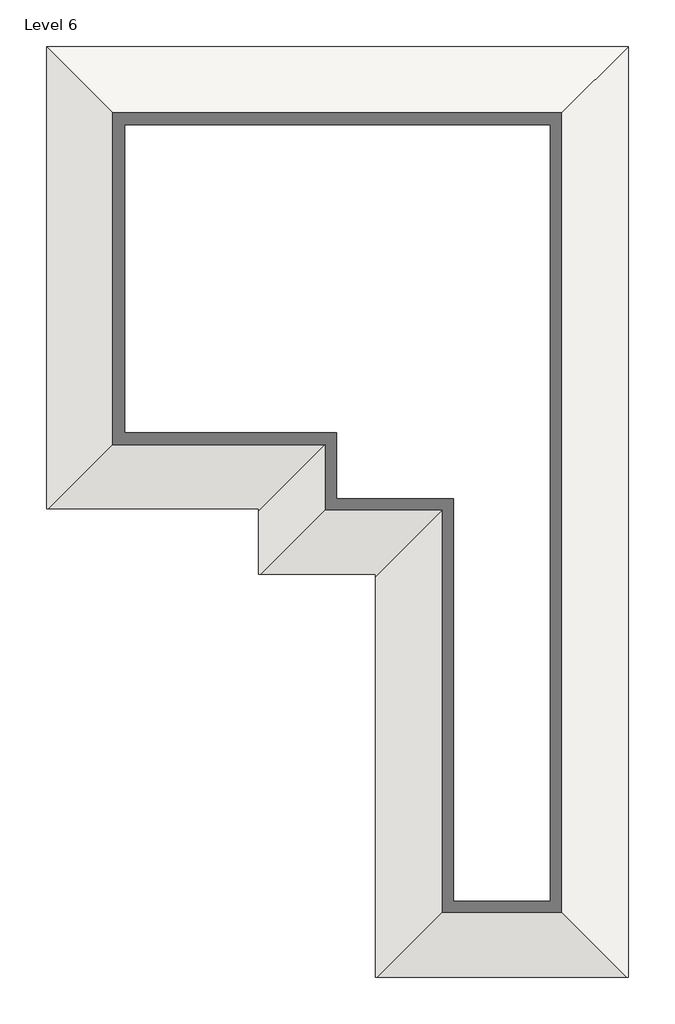
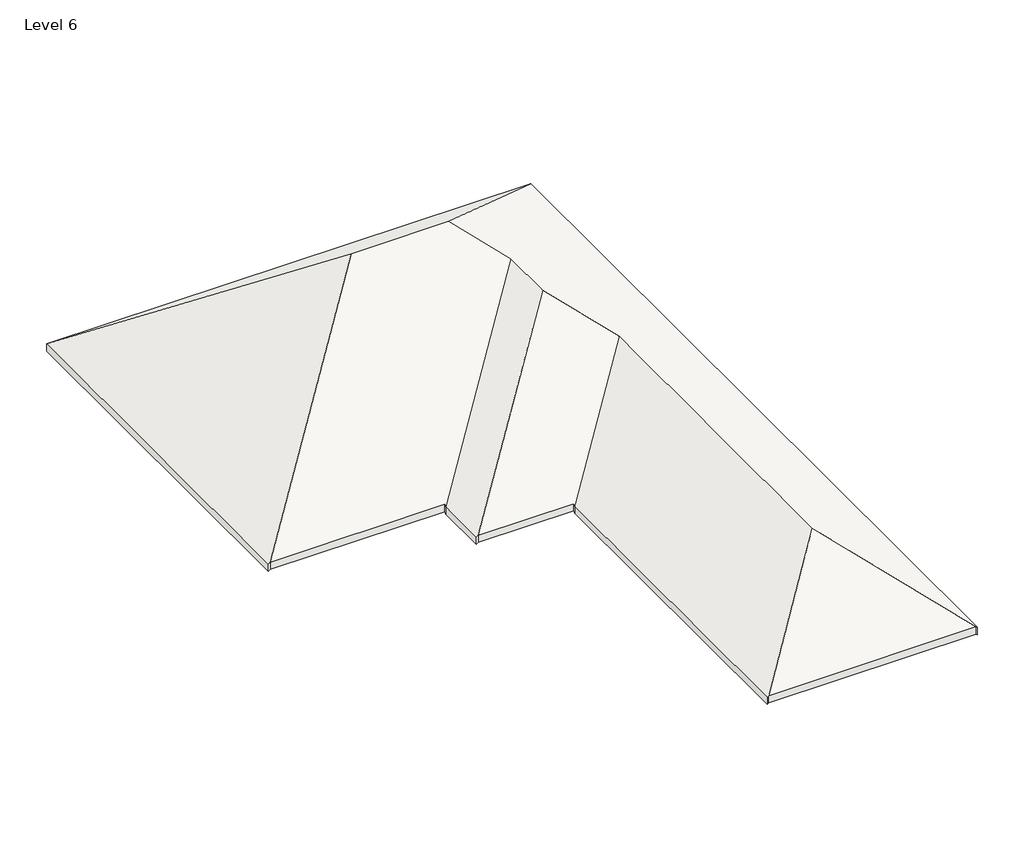
# One storey: 1 roof.
"""IFC4 building model written with IfcOpenShell, lengths in millimetres."""

from ifc_helpers import new_model, si_unit, origin, place, context, project, spatial, faceted_brep, element, save

model = new_model("IFC4")

# Units and contexts
model_context = context("Model", 3, world=origin())
ifc_project = project(units=[si_unit("LENGTHUNIT", "METRE", prefix="MILLI")], contexts=[model_context])

# Site, building, storey
site = spatial("IfcSite", under=ifc_project)
building = spatial("IfcBuilding", under=site)
storey = spatial("IfcBuildingStorey", under=building, Name="Level 6", Elevation=11233.15)

# Roof
placement = place(None, origin())
element("IfcRoof", 1, ObjectType="6\" 2", at=placement, inside=storey, context=model_context, shape_type="Brep", body=[
    faceted_brep([(-14235.3059085, 14471.5414483, 11204.575), (-9396.6059085, 9632.8414483, 14833.6), (-14184.5059085, 4844.9414483, 11242.675), (-14235.3059085, 4844.9414483, 11204.575), (-2106.8059085, 14471.5414483, 11204.575), (-2106.8059085, -4921.3585517, 11204.575), (-2144.9059085, -4921.3585517, 11233.15), (-4742.0559085, -2324.2085517, 13181.0125), (-4742.0559085, 6057.7914483, 13181.0125), (-5961.2559085, 7276.9914483, 14095.4125), (-5961.2559085, 8648.5914483, 14095.4125), (-6945.5059085, 9632.8414483, 14833.6), (-14235.3059085, 14471.5414483, 11395.075), (-14235.3059085, 4844.9414483, 11395.075), (-14184.5059085, 4844.9414483, 11433.175), (-9396.6059085, 9632.8414483, 15024.1), (-2106.8059085, 14471.5414483, 11395.075), (-6945.5059085, 9632.8414483, 15024.1), (-5961.2559085, 8648.5914483, 14285.9125), (-5961.2559085, 7276.9914483, 14285.9125), (-4742.0559085, 6057.7914483, 13371.5125), (-4742.0559085, -2324.2085517, 13371.5125), (-2144.9059085, -4921.3585517, 11423.65), (-2106.8059085, -4921.3585517, 11395.075), (-9815.7059085, 4794.1414483, 11395.075), (-9815.7059085, 4844.9414483, 11433.175), (-9815.7059085, 4844.9414483, 11242.675), (-9815.7059085, 4794.1414483, 11204.575), (-9764.9059085, 3473.3414483, 11433.175), (-9815.7059085, 3473.3414483, 11395.075), (-9815.7059085, 3473.3414483, 11204.575), (-9764.9059085, 3473.3414483, 11242.675), (-7377.3059085, 3422.5414483, 11395.075), (-7377.3059085, 3473.3414483, 11433.175), (-7377.3059085, 3473.3414483, 11242.675), (-7377.3059085, 3422.5414483, 11204.575), (-7339.2059085, -4921.3585517, 11233.15), (-7377.3059085, -4921.3585517, 11204.575), (-7339.2059085, -4921.3585517, 11423.65), (-7377.3059085, -4921.3585517, 11395.075)], [[[0, 1, 2, 3]], [[4, 5, 6, 7, 8, 9, 10, 11]], [[4, 11, 1, 0]], [[12, 13, 14, 15]], [[16, 17, 18, 19, 20, 21, 22, 23]], [[16, 12, 15, 17]], [[0, 12, 16, 4]], [[3, 13, 12, 0]], [[4, 16, 23, 5]], [[14, 13, 3, 2]], [[24, 25, 26, 27]], [[28, 29, 30, 31]], [[32, 33, 34, 35]], [[2, 1, 11, 10, 27, 26]], [[36, 7, 6]], [[27, 10, 9, 31, 30]], [[31, 9, 8, 35, 34]], [[35, 8, 7, 36, 37]], [[14, 25, 24, 18, 17, 15]], [[38, 22, 21]], [[24, 29, 28, 19, 18]], [[28, 33, 32, 20, 19]], [[32, 39, 38, 21, 20]], [[26, 25, 14, 2]], [[30, 29, 24, 27]], [[34, 33, 28, 31]], [[37, 39, 32, 35]], [[6, 22, 38, 36]], [[38, 39, 37, 36]], [[23, 22, 6, 5]]]),
])

save(model, "model.ifc")

# Revit data of these elements
# Type "6\" 2"
#   Assembly Code = "B1020"
#   Layers, outside or top first: 0' - 6" "roof" (function 1)
# Element 1 (IfcRoof, "6\" 2")
#   built-in parameter 1001705 = 49.2917 (stored number, unit not read)
#   built-in parameter 1001710 = 33615
#   Phase Created = New Construction
#   Materials on its faces: "roof"
# Materials
#   "roof": class "Generic", colour RGB 120 120 120, transparency 0, Cost = 0
